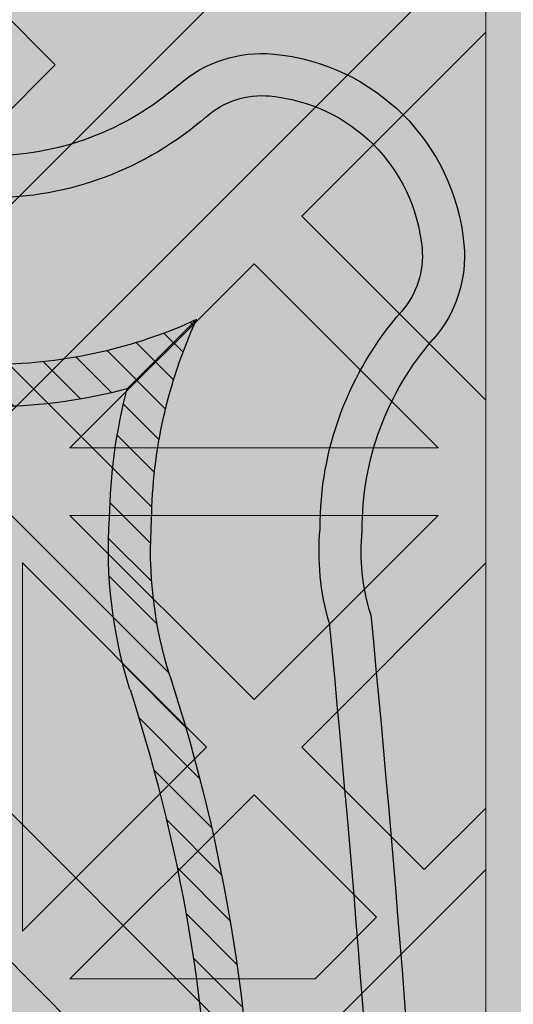
# Model space of a CAD drawing. Units: inches. Extents: x 844 to 2234, y 346 to 1084.
# Tile 86 of 93: x 2006.557 to 2008.425, y 706.497 to 710.224. Entities that reach past the tile are written whole.
import ezdxf

# ---------------------------------------------------------------- set-up
doc = ezdxf.new("R2010")
doc.units = ezdxf.units.IN
doc.header["$MEASUREMENT"] = 0
for name, color, linetype, lineweight in [('A-ANNO-DIMS', 2, 'Continuous', 18), ('furniture', 8, 'Continuous', 18), ('RA-AP-01$0$INT', 35, 'Continuous', 5)]:
    doc.layers.add(name, color=color, linetype=linetype, lineweight=lineweight)
doc.layers.add('RA-AP-01$0$FURN', color=3, linetype='Continuous')
doc.layers.add('RA-AP-01$0$WOOD', color=64, linetype='Continuous')
doc.styles.get("Standard").update_dxf_attribs({"font": 'arial.ttf'})
doc.dimstyles.get("Standard").update_dxf_attribs({"dimtxt": 6, "dimasz": 3, "dimexe": 0.18, "dimexo": 0.0625, "dimgap": 0.09, "dimtad": 0, "dimtih": 1, "dimtoh": 1, "dimdec": 1, "dimzin": 0, "dimdsep": 46, "dimlunit": 3, "dimtxsty": 'Standard', "dimblk": 'ARCHTICK', "dimcen": 0.09, "dimadec": 0, "dimazin": 0, "dimtfac": 1, "dimtdec": 1, "dimtofl": 0, "dimtmove": 0, "dimatfit": 3, "dimfxl": 1, "dimtolj": 1, "dimtzin": 0, "dimarcsym": 0})

# ---------------------------------------------------------------- blocks, each defined once
blk = doc.blocks.new('A$C18D01794')
at = {"layer": 'RA-AP-01$0$INT'}
blk.add_hatch(color=256, dxfattribs=at).paths.add_polyline_path([(4.505206456958071, -7.906712009588039), (5.305206456958072, -7.906712009588039), (5.305206456958072, -7.106712009588038), (5.255206456951893, -7.106712009588036), (5.25520645694868, -7.856712009570104), (4.555206456959269, -7.856712009588616), (4.555206456956052, -7.106712009588038), (4.505206456958073, -7.106712009588038)])
h = blk.add_hatch(color=256, dxfattribs=at)
h.paths.add_polyline_path([(4.585917135068448, -7.856712009587804), (4.614201406330596, -7.856712009587056), (4.668846067270487, -7.802067348644738), (4.723490728212344, -7.856712009584164), (4.771774999457151, -7.856712009582887), (4.826419660396886, -7.80206734864072), (4.862780050090322, -7.838427738332541), (4.844495778842715, -7.856712009580965), (4.862780050090411, -7.856712009580482), (4.905206456960182, -7.814285602707865), (4.947632863832445, -7.856712009578238), (4.965917135079675, -7.856712009577755), (4.947632863831759, -7.838427738330656), (4.983993253523576, -7.802067348637219), (5.038637914464627, -7.856712009575829), (5.08692218571208, -7.856712009574554), (5.141566846649976, -7.802067348634224), (5.196211507589851, -7.856712009571666), (5.224495778822615, -7.856712009570916), (4.905206456953975, -7.537422687702283)])
h.paths.add_polyline_path([(4.895206456956031, -7.575706958950402), (4.895206456958921, -7.684996280828174), (4.840561796018589, -7.630351619890275)], flags=16)
h.paths.add_polyline_path([(4.915206456955638, -7.575706958949956), (4.969851117895509, -7.630351619887399), (4.915206456957609, -7.684996280827732)], flags=16)
h.paths.add_polyline_path([(4.826419660395175, -7.644493755514321), (4.881064321335613, -7.699138416452331), (4.771774999456703, -7.69913841645522)], flags=16)
h.paths.add_polyline_path([(4.983993253519558, -7.644493755510815), (5.038637914460456, -7.699138416449285), (4.929348592581548, -7.69913841645126)], flags=16)
h.paths.add_polyline_path([(4.881064321336025, -7.719138416452334), (4.826419660397532, -7.773783077393256), (4.771774999457062, -7.719138416455217)], flags=16)
h.paths.add_polyline_path([(4.929348592582019, -7.71913841645126), (5.038637914460982, -7.719138416449284), (4.983993253522945, -7.773783077389749)], flags=16)
h.paths.add_polyline_path([(4.895206456960191, -7.733280552075633), (4.895206456962115, -7.806001331460164), (4.876922185715016, -7.824285602708492), (4.840561796021581, -7.787925213016675)], flags=16)
h.paths.add_polyline_path([(4.915206456958487, -7.733280552075187), (4.969851117899527, -7.787925213013798), (4.933490728206909, -7.824285602708034), (4.9152064569598, -7.806001331461736)], flags=16)
h.paths.add_polyline_path([(4.757632863832376, -7.733280552079264), (4.812277524772842, -7.787925213017304), (4.757632863834348, -7.842569873958233)], flags=16)
h.paths.add_polyline_path([(4.737632863832376, -7.73328055207979), (4.737632863834348, -7.842569873958701), (4.682988202893906, -7.787925213020692)], flags=16)
h.paths.add_polyline_path([(5.05278005008503, -7.733280552072701), (5.052780050087917, -7.842569873951664), (4.998135389146995, -7.787925213013169)], flags=16)
h.paths.add_polyline_path([(5.072780050085024, -7.733280552072333), (5.127424711025931, -7.787925213010806), (5.072780050087916, -7.842569873951244)], flags=16)
h.paths.add_polyline_path([(4.935917135072783, -7.506712009583784), (5.255206456948811, -7.826001331459767), (5.255206456948932, -7.797717060211899), (5.200561796010279, -7.743072399273238), (5.255206456949403, -7.688427738334128), (5.25520645694961, -7.640143467086677), (5.200561796009787, -7.585498806146837), (5.236922185702417, -7.549138416454212), (5.255206456949919, -7.56742268770172), (5.255206456949998, -7.549138416454178), (5.212780050078687, -7.506712009583814), (5.25520645695036, -7.464285602712145), (5.255206456950438, -7.446001331464763), (5.236922185702424, -7.464285602712779), (5.200561796009796, -7.427925213020149), (5.255206456950753, -7.373280552079203), (5.25520645695096, -7.324996280834394), (5.200561796010322, -7.270351619893748), (5.255206456951428, -7.215706958952649), (5.255206456951547, -7.187422687705071)])
h.paths.add_polyline_path([(5.042988202883395, -7.42792521302065), (5.097632863823085, -7.373280552080975), (5.097632863822622, -7.482569873959883)], flags=16)
h.paths.add_polyline_path([(5.028846067259663, -7.442067348644384), (5.083490728198774, -7.496712009583504), (4.974201406321001, -7.496712009583035)], flags=16)
h.paths.add_polyline_path([(5.117632863823087, -7.37328055208089), (5.172277524762331, -7.42792521302015), (5.11763286382262, -7.482569873959851)], flags=16)
h.paths.add_polyline_path([(5.08349072819877, -7.516712009582191), (5.028846067259652, -7.571356670521302), (4.974201406320998, -7.516712009582638)], flags=16)
h.paths.add_polyline_path([(5.131774999446817, -7.35913841645716), (5.186419660386065, -7.413783077396415), (5.241064321325782, -7.359138416456712)], flags=17)
h.paths.add_polyline_path([(5.131774999446228, -7.496712009583703), (5.186419660386065, -7.442067348643883), (5.222780050079488, -7.478427738337313), (5.204495778832781, -7.496712009584014)], flags=16)
h.paths.add_polyline_path([(5.097632863822613, -7.530854145205813), (5.097632863823061, -7.640143467084723), (5.042988202883383, -7.585498806145032)], flags=16)
h.paths.add_polyline_path([(5.131774999446899, -7.339138416457162), (5.241064321325809, -7.339138416456712), (5.186419660386591, -7.284493755517479)], flags=17)
h.paths.add_polyline_path([(5.131774999446226, -7.516712009581999), (5.204495778830767, -7.516712009581702), (5.22278005007868, -7.534996280829206), (5.186419660386049, -7.571356670521828)], flags=16)
h.paths.add_polyline_path([(5.11763286382262, -7.530854145205852), (5.17227752476232, -7.585498806145562), (5.117632863823064, -7.64014346708481)], flags=16)
h.paths.add_polyline_path([(5.186419660386069, -7.599640941770585), (5.241064321325754, -7.654285602710281), (5.131774999446791, -7.654285602709814)], flags=16)
h.paths.add_polyline_path([(5.131774999446872, -7.674285602709813), (5.24106432132578, -7.674285602710282), (5.186419660386554, -7.728930263649504)], flags=16)
h.paths.add_polyline_path([(5.255206456951811, -7.126001331467467), (5.255206456951895, -7.106712009588038), (4.555206456956052, -7.106712009588038), (4.555206456956136, -7.12600133146746), (4.905206456953973, -7.476001331465289)])
h.paths.add_polyline_path([(4.983993253513404, -7.368930263651977), (4.92934859257295, -7.314285602713969), (5.03863791445186, -7.314285602711063)], flags=16)
h.paths.add_polyline_path([(4.969851117889988, -7.383072399276016), (4.915206456952556, -7.437717060215906), (4.915206456949648, -7.328427738338133)], flags=16)
h.paths.add_polyline_path([(4.929348592572535, -7.294285602713971), (4.983993253511019, -7.239640941773039), (5.038637914451496, -7.294285602711065)], flags=16)
h.paths.add_polyline_path([(5.052780050074912, -7.280143467087016), (4.998135389134438, -7.225498806148989), (5.052780050072919, -7.170854145208052)], flags=16)
h.paths.add_polyline_path([(5.07278005007491, -7.280143467086489), (5.072780050072918, -7.170854145207579), (5.127424711013374, -7.225498806145578)], flags=16)
h.paths.add_polyline_path([(4.89520645695295, -7.437717060216355), (4.840561796013067, -7.383072399278919), (4.895206456950961, -7.328427738338582)], flags=16)
h.paths.add_polyline_path([(4.915206456948365, -7.280143467090674), (4.915206456946434, -7.207422687704125), (4.933490728192729, -7.18913841645701), (4.969851117886972, -7.225498806149623)], flags=16)
h.paths.add_polyline_path([(4.881064321327021, -7.314285602715054), (4.82641966038902, -7.368930263655506), (4.771774999448108, -7.314285602717047)], flags=16)
h.paths.add_polyline_path([(4.895206456950073, -7.280143467091125), (4.840561796009022, -7.225498806152518), (4.876922185700835, -7.18913841645908), (4.895206456948749, -7.207422687706589)], flags=16)
h.paths.add_polyline_path([(4.983993253510392, -7.211356670525576), (4.947632863816944, -7.174996280833758), (4.965917135064043, -7.156712009585847), (5.038637914448995, -7.156712009584522)], flags=16)
h.paths.add_polyline_path([(4.881064321326543, -7.294285602715056), (4.771774999447578, -7.294285602717046), (4.826419660385607, -7.239640941776569)], flags=16)
h.paths.add_polyline_path([(4.905206456946447, -7.19913841645844), (4.862780050074785, -7.156712009587725), (4.947632863816685, -7.156712009586302)], flags=16)
h.paths.add_polyline_path([(5.14156684663679, -7.211356670521528), (5.086922185696452, -7.156712009583639), (5.196211507574223, -7.156712009581651)], flags=16)
h.paths.add_polyline_path([(4.8264196603837, -7.211356670529104), (4.771774999442643, -7.156712009590501), (4.8444957788276, -7.156712009588568), (4.862780050075511, -7.17499628083566)], flags=16)
h.paths.add_polyline_path([(4.812277524760289, -7.225498806153156), (4.757632863822258, -7.28014346709363), (4.757632863819352, -7.170854145214669)], flags=16)
h.paths.add_polyline_path([(4.73763286382226, -7.280143467093997), (4.682988202881349, -7.22549880615554), (4.737632863819352, -7.170854145215086)], flags=16)
h.paths.add_polyline_path([(4.723490728195188, -7.156712009591787), (4.668846067257299, -7.211356670532127), (4.614201406317417, -7.156712009594693)], flags=16)
h.paths.add_polyline_path([(4.597632863829262, -7.506712009583814), (4.555206456957951, -7.54913841645418), (4.555206456958029, -7.56742268770172), (4.573490728205535, -7.549138416454212), (4.609851117898167, -7.585498806146839), (4.555206456958338, -7.640143467086675), (4.555206456958546, -7.688427738334125), (4.60985111789767, -7.743072399273238), (4.555206456959015, -7.797717060211899), (4.555206456959138, -7.826001331459767), (4.874495778835167, -7.506712009583786), (4.5552064569564, -7.187422687705062), (4.555206456956523, -7.215706958952644), (4.609851117897629, -7.270351619893746), (4.555206456956988, -7.324996280834396), (4.555206456957198, -7.373280552079195), (4.609851117898153, -7.427925213020147), (4.573490728205528, -7.464285602712779), (4.555206456957507, -7.446001331464756), (4.555206456957585, -7.464285602712143)])
h.paths.add_polyline_path([(4.712780050085332, -7.482569873959882), (4.712780050084863, -7.373280552080972), (4.767424711024555, -7.42792521302065)], flags=16)
h.paths.add_polyline_path([(4.726922185709173, -7.496712009583504), (4.781566846648288, -7.442067348644384), (4.836211507586949, -7.496712009583033)], flags=16)
h.paths.add_polyline_path([(4.692780050085327, -7.482569873959851), (4.638135389145619, -7.427925213020149), (4.692780050084865, -7.373280552080892)], flags=16)
h.paths.add_polyline_path([(4.726922185709182, -7.516712009582191), (4.836211507586949, -7.51671200958264), (4.7815668466483, -7.571356670521304)], flags=16)
h.paths.add_polyline_path([(4.678637914461726, -7.496712009583706), (4.605917135075169, -7.496712009584014), (4.587632863828464, -7.478427738337311), (4.623993253521887, -7.442067348643881)], flags=16)
h.paths.add_polyline_path([(4.712780050085336, -7.530854145205816), (4.767424711024568, -7.585498806145034), (4.71278005008489, -7.640143467084724)], flags=16)
h.paths.add_polyline_path([(4.678637914461726, -7.516712009582001), (4.623993253521899, -7.571356670521829), (4.587632863829271, -7.534996280829206), (4.605917135077185, -7.5167120095817)], flags=16)
h.paths.add_polyline_path([(4.692780050085336, -7.530854145205848), (4.692780050084889, -7.64014346708481), (4.638135389145632, -7.585498806145562)], flags=16)
h.paths.add_polyline_path([(4.623993253521885, -7.413783077396415), (4.678637914461131, -7.359138416457161), (4.56934859258217, -7.359138416456712)], flags=17)
h.paths.add_polyline_path([(4.623993253521901, -7.599640941770568), (4.678637914461158, -7.654285602709814), (4.569348592582195, -7.654285602710281)], flags=16)
h.paths.add_polyline_path([(4.678637914461051, -7.339138416457162), (4.623993253521361, -7.284493755517479), (4.569348592582143, -7.339138416456712)], flags=17)
h.paths.add_polyline_path([(4.678637914461076, -7.674285602709813), (4.623993253521399, -7.728930263649504), (4.569348592582167, -7.674285602710281)], flags=16)
h = blk.add_hatch(color=256, dxfattribs=at)
h.paths.add_polyline_path([(4.905206456954232, -7.537422687702028), (4.874495778835232, -7.506712009583718), (4.555206456959138, -7.826001331459766), (4.555206456959269, -7.856712009588616), (4.585917135068449, -7.856712009587804)])
h.paths.add_polyline_path([(4.935917135072152, -7.506712009583152), (4.905206456953497, -7.537422687701806), (5.224495778822614, -7.856712009570917), (5.255206456948681, -7.856712009570104), (5.255206456948813, -7.826001331459768)])
h.paths.add_polyline_path([(5.255206456951549, -7.18742268770507), (5.255206456951813, -7.126001331467461), (4.905206456953563, -7.476001331465701), (4.935917135072559, -7.506712009584006)])
h.paths.add_polyline_path([(4.874495778835167, -7.506712009583785), (4.905206456953818, -7.476001331465132), (4.555206456956135, -7.126001331467458), (4.555206456956399, -7.187422687705064)])
h = blk.add_hatch(color=256, dxfattribs=at)
h.paths.add_polyline_path([(4.781566846647504, -7.442067348645805), (4.836211507586161, -7.496712009584463), (4.726922185708388, -7.496712009584918)])
h.paths.add_polyline_path([(4.836211507586161, -7.516712009584068), (4.781566846647504, -7.571356670522723), (4.726922185708388, -7.516712009583606)])
h.paths.add_polyline_path([(4.76742471102377, -7.585498806146453), (4.712780050084083, -7.640143467086137), (4.712780050084542, -7.530854145207227)])
h.paths.add_polyline_path([(4.692780050084544, -7.530854145207257), (4.692780050084084, -7.64014346708622), (4.638135389144834, -7.585498806146965)])
h.paths.add_polyline_path([(4.678637914460932, -7.516712009583407), (4.623993253521102, -7.571356670523233), (4.587632863827676, -7.53499628082981), (4.605917135074382, -7.516712009583104)])
h.paths.add_polyline_path([(4.573490728204743, -7.54913841645434), (4.60985111789737, -7.585498806146969), (4.555206456957541, -7.640143467086797), (4.555206456957237, -7.567422687701846)])
h.paths.add_polyline_path([(4.623993253521098, -7.599640941770699), (4.67863791446035, -7.654285602709951), (4.56934859258139, -7.654285602710407)])
h.paths.add_polyline_path([(4.678637914460275, -7.67428560270995), (4.623993253520583, -7.728930263649637), (4.56934859258136, -7.674285602710405)])
h.paths.add_polyline_path([(4.609851117896854, -7.743072399273369), (4.555206456958196, -7.797717060212026), (4.555206456957738, -7.688427738334254)])
h.paths.add_polyline_path([(4.597632863828475, -7.506712009583301), (4.555206456957283, -7.549138416454495), (4.555206456956805, -7.464285602712587)])
h.paths.add_polyline_path([(4.678637914460932, -7.496712009585113), (4.605917135076396, -7.496712009585417), (4.587632863828479, -7.478427738337913), (4.623993253521104, -7.442067348645284)])
h.paths.add_polyline_path([(4.692780050084091, -7.373280552082301), (4.692780050084548, -7.482569873961267), (4.638135389144834, -7.427925213021552)])
h.paths.add_polyline_path([(4.767424711023772, -7.427925213022072), (4.712780050084545, -7.48256987396129), (4.712780050084089, -7.373280552082384)])
h.paths.add_polyline_path([(4.67863791446036, -7.359138416457298), (4.623993253521105, -7.41378307739655), (4.569348592581399, -7.35913841645684)])
h.paths.add_polyline_path([(4.609851117897371, -7.427925213020278), (4.573490728204743, -7.464285602712907), (4.555206456957237, -7.446001331465401), (4.555206456957548, -7.373280552080448)])
h.paths.add_polyline_path([(4.623993253520596, -7.284493755517612), (4.67863791446028, -7.339138416457299), (4.569348592581367, -7.339138416456838)])
h.paths.add_polyline_path([(4.609851117896867, -7.270351619893878), (4.555206456957749, -7.324996280832994), (4.55520645695821, -7.21570695895522)])
h = blk.add_hatch(color=256, dxfattribs=at)
h.paths.add_polyline_path([(4.969851117891331, -7.630351619889621), (4.915206456952669, -7.575706958950966), (4.915206456952222, -7.684996280828739)])
h.paths.add_polyline_path([(4.895206456953064, -7.575706958950968), (4.840561796014413, -7.630351619889628), (4.895206456953533, -7.684996280828741)])
h.paths.add_polyline_path([(4.826419660390684, -7.644493755513362), (4.771774999451003, -7.699138416453052), (4.881064321329913, -7.699138416452587)])
h.paths.add_polyline_path([(4.881064321329884, -7.719138416452585), (4.771774999450921, -7.719138416453052), (4.82641966039018, -7.773783077392298)])
h.paths.add_polyline_path([(4.895206456953734, -7.733280552076196), (4.840561796013912, -7.787925213016031), (4.876922185707337, -7.824285602709455), (4.895206456954043, -7.806001331462747)])
h.paths.add_polyline_path([(4.862780050082808, -7.838427738332388), (4.826419660390178, -7.802067348639763), (4.771774999450351, -7.856712009579595), (4.844495778835303, -7.856712009579895)])
h.paths.add_polyline_path([(4.812277524766446, -7.787925213016036), (4.757632863827191, -7.733280552076788), (4.757632863826741, -7.842569873955747)])
h.paths.add_polyline_path([(4.737632863827191, -7.733280552076863), (4.682988202887508, -7.787925213016558), (4.737632863826743, -7.842569873955778)])
h.paths.add_polyline_path([(4.668846067263777, -7.802067348640287), (4.614201406325123, -7.856712009578949), (4.723490728202894, -7.856712009579402)])
h.paths.add_polyline_path([(4.905206456953846, -7.814285602708654), (4.862780050082654, -7.856712009579847), (4.947632863824561, -7.85671200958032)])
h.paths.add_polyline_path([(4.915206456952028, -7.733280552076195), (4.91520645695173, -7.806001331460731), (4.933490728199234, -7.824285602708648), (4.96985111789186, -7.787925213016022)])
h.paths.add_polyline_path([(5.038637914454841, -7.719138416453029), (4.929348592575874, -7.71913841645258), (4.983993253515593, -7.773783077392289)])
h.paths.add_polyline_path([(4.983993253515065, -7.644493755513352), (4.929348592575849, -7.699138416452582), (5.038637914454755, -7.699138416453031)])
h.paths.add_polyline_path([(5.052780050079843, -7.73328055207676), (4.998135389140595, -7.787925213016018), (5.052780050080309, -7.842569873955721)])
h.paths.add_polyline_path([(4.983993253516868, -7.802067348639752), (4.947632863824241, -7.838427738332383), (4.965917135071747, -7.856712009579888), (5.038637914456701, -7.856712009579572)])
h.paths.add_polyline_path([(5.127424711019533, -7.787925213016519), (5.072780050079843, -7.733280552076838), (5.07278005008031, -7.842569873955751)])
h.paths.add_polyline_path([(5.141566846643269, -7.802067348640248), (5.086922185704154, -7.85671200957937), (5.196211507581929, -7.856712009578901)])
for p, q in [((4.555206456956052, -7.106712009588036), (4.555206456959269, -7.856712009588616)), ((4.55520645695807, -7.464285602712626), (4.555206456957598, -7.549138416454534)), ((4.597632863829264, -7.506712009583814), (4.555206456957598, -7.549138416454534)), ((4.874495778835167, -7.506712009583786), (4.555206456959136, -7.826001331459769)), ((4.605917135074869, -7.516712009584017), (4.587632863829269, -7.534996280829206)), ((4.605917135076771, -7.5167120095817), (4.678637914461723, -7.516712009581999)), ((4.678637914461723, -7.516712009581999), (4.623993253521898, -7.571356670521829)), ((4.692780050085336, -7.530854145205847), (4.638135389145632, -7.585498806145562)), ((4.692780050084889, -7.64014346708481), (4.692780050085336, -7.530854145205847)), ((4.623993253521899, -7.571356670521829), (4.587632863829269, -7.534996280829206)), ((4.905206456953975, -7.537422687702283), (4.585917135071132, -7.856712009585121)), ((4.555206456958031, -7.56742268770172), (4.573490728205535, -7.549138416454212)), ((4.609851117898167, -7.585498806146839), (4.573490728205535, -7.549138416454214)), ((4.555206456958033, -7.56742268770172), (4.555206456958345, -7.640143467086671)), ((4.555206456958345, -7.640143467086671), (4.609851117898167, -7.585498806146837)), ((4.692780050084889, -7.64014346708481), (4.638135389145632, -7.585498806145562)), ((4.569348592582195, -7.654285602710281), (4.623993253521901, -7.599640941770568)), ((4.678637914461158, -7.654285602709814), (4.623993253521901, -7.599640941770568)), ((4.678637914461158, -7.654285602709814), (4.569348592582195, -7.654285602710281)), ((4.569348592582168, -7.674285602710281), (4.623993253521399, -7.728930263649504)), ((4.678637914461078, -7.674285602709813), (4.569348592582168, -7.674285602710281)), ((4.6239932535214, -7.728930263649502), (4.678637914461078, -7.674285602709813)), ((4.555206456958551, -7.68842773833413), (4.60985111789767, -7.743072399273238)), ((4.682988202893908, -7.78792521302069), (4.737632863832376, -7.733280552079792)), ((4.555206456959017, -7.797717060211899), (4.60985111789767, -7.743072399273238)), ((4.737632863834348, -7.842569873958701), (4.682988202893906, -7.787925213020692))]:
    blk.add_line(p, q, dxfattribs=at)
blk = doc.blocks.new('A$C32926AE1')
at = {"layer": 'RA-AP-01$0$WOOD'}
h = blk.add_hatch(color=256, dxfattribs=at)
h.dxf.hatch_style = 1
h.paths.add_polyline_path([(5.157430609644524, 4.573483066760929, -0.1009492694046607), (5.155401577623758, 4.593365984175333, -0.1842662638101597), (5.172249623284174, 4.638795604568598, 0.2056608120311276), (5.179560981299304, 4.661316324430096, 0.3614336704623542), (5.134352340494423, 4.706524965234944, 0.2056608120311297), (5.111831620632933, 4.699213607219793, -0.1842662638101113), (5.066402000239693, 4.682365561559342, -0.1055311479399994), (5.045656153913092, 4.68467289944697, 0.1567636581983829), (4.763886414745334, 4.684672899446966, -0.1055311479399895), (4.743140568418733, 4.68236556155934, -0.1842662638100833), (4.6977109480255, 4.69921360721979, 0.2056608120302612), (4.675190228164109, 4.706524965234949, 0.3614336704708441), (4.629981587358889, 4.66131632442871, 0.2056608120245944), (4.637292945374126, 4.638795604567974, -0.1842662638101024), (4.654140991034615, 4.59336598417475, -0.1009492694055169), (4.652111959013835, 4.573483066760181, 0.021410119221476), (4.629748025606143, 4.156712009541676, 0.0214101192214795), (4.652111959013809, 3.739940952323101, -0.1009492694059586), (4.654140991034615, 3.720058034908448, -0.1842662638100975), (4.637292945374126, 3.674628414515226, 0.2056608120245705), (4.629981587358889, 3.652107694654492, 0.3614336704708879), (4.675190228164113, 3.606899053848249, 0.2056608120302384), (4.697710948025501, 3.614210411863408, -0.1842662638100995), (4.743140568418738, 3.63105845752386, -0.1055311479402541), (4.763886414745388, 3.628751119636215, 0.1567636581983776), (5.045656153913137, 3.628751119636244, -0.1055311479397538), (5.066402000239692, 3.631058457523857, -0.1842662638101067), (5.111831620632931, 3.614210411863407, 0.2056608120310924), (5.134352340494417, 3.606899053848256, 0.3614336704624001), (5.179560981299307, 3.652107694653103, 0.2056608120311314), (5.172249623284175, 3.6746284145146, -0.1842662638101402), (5.155401577623758, 3.72005803490786, -0.1009492694051366), (5.15743060964455, 3.739940952322354, 0.0214101192215073), (5.179794543052287, 4.156712009541468, 0.0214101192215252)])
h.paths.add_polyline_path([(4.639748609479751, 4.156712009541513, 0.0213537860821624), (4.661970494867118, 3.741887061152232, -0.094075836301374), (4.664143710413708, 3.7196126951003, -0.1824818158568985), (4.644813765429836, 3.668037719127816, 0.2056608120245319), (4.639939526753007, 3.653023905887301, 0.3614336704710246), (4.676106439397173, 3.616856993242342, 0.2056608120302234), (4.691120252638095, 3.621731231919122, -0.1824818158602558), (4.742695228611606, 3.641061176902986, -0.1029891339458722), (4.766991894714349, 3.638256818950944, 0.156709409989566), (5.042550673941472, 3.638256818950105, -0.102989133958497), (5.066847340047078, 3.641061176902949, -0.1824818158594995), (5.118422316020358, 3.621731231919103, 0.2056608120311416), (5.133436129261316, 3.616856993242346, 0.3614336704621468), (5.169603041905217, 3.653023905886178, 0.2056608120310986), (5.164728803228477, 3.668037719127177, -0.1824818158565612), (5.145398858244737, 3.719612695099578, -0.0940758363009313), (5.147572073791232, 3.741887061151398, 0.0213537860822023), (5.169793959178681, 4.156712009541451, 0.0213537860822226), (5.147572073791203, 4.571536957931898, -0.0940758363005034), (5.145398858244737, 4.59381132398362, -0.1824818158565587), (5.164728803228476, 4.645386299956021, 0.2056608120311045), (5.169603041905216, 4.66040011319702, 0.3614336704621845), (5.133436129261313, 4.696567025840856, 0.2056608120310773), (5.118422316020359, 4.691692787164098, -0.182481815859508), (5.066847340047078, 4.67236284218025, -0.1029891339584606), (5.04255067394148, 4.675167200133092, 0.156709409989566), (4.766991894714357, 4.675167200132257, -0.1029891339458842), (4.742695228611611, 4.672362842180213, -0.1824818158602725), (4.691120252638095, 4.691692787164077, 0.2056608120302152), (4.676106439397174, 4.696567025840858, 0.3614336704710363), (4.639939526753005, 4.660400113195899, 0.2056608120245495), (4.644813765429837, 4.645386299955384, -0.1824818158568934), (4.664143710413708, 4.593811323982902, -0.0940758363009187), (4.661970494867149, 4.571536957931074, 0.021353786082177)], flags=16)
h.paths.add_polyline_path([(5.129794543052235, 4.432167055276933, -0.0141661062790638), (5.130152669293814, 4.156927903047693, -0.0141661062790647), (5.129794543052234, 3.881688750818433, -0.0785247771143638), (5.10979738006795, 3.755143611847103, 0.0945969212073497), (5.105408519571111, 3.717898134952927, 0.1043170707844957), (5.116074640131521, 3.670385395016088, 0.1043170707864965), (5.068561900193738, 3.681051515576561, 0.09459692119553), (5.031316423304057, 3.676662655080835, -0.1580239521427272), (4.778226145355827, 3.676662655080367, 0.0945969211986668), (4.740980668464973, 3.681051515576592, 0.1043170707882822), (4.693467928526415, 3.670385395015844, 0.1043170707867916), (4.704134049087309, 3.717898134953662, 0.0945969211972894), (4.69974518859162, 3.755143611844042, -0.0785247771163196), (4.679748025606343, 3.881688750818406, -0.0141661062790663), (4.679389899364763, 4.156927903047693, -0.0141661062790672), (4.679748025606343, 4.432167055276998, -0.0785247771163064), (4.699745188591625, 4.55871219425134, 0.094596921197333), (4.704134049087308, 4.595957671141738, 0.1043170707867205), (4.693467928526416, 4.643470411079523, 0.1043170707882628), (4.740980668464965, 4.632804290518776, 0.0945969211988114), (4.778226145355874, 4.637193151015016, -0.158023952142669), (5.031316423304015, 4.637193151014546, 0.0945969211956361), (5.068561900193736, 4.632804290518806, 0.1043170707864979), (5.11607464013152, 4.643470411079278, 0.1043170707844617), (5.105408519571112, 4.595957671142455, 0.0945969212074597), (5.109797380067959, 4.558712194248236, -0.0785247771143467)], flags=0)
h.paths.add_polyline_path([(5.119794532311105, 4.432259799204851, -0.0142000800617244), (5.120156169157484, 4.156927903047701, -0.0142000800617277), (5.119794532311105, 3.881596006890482, -0.0784894509520253), (5.100273383573699, 3.758192358677797, 0.0940138827242913), (5.095413455884425, 3.717477693979438, 0.0606271852308753), (5.099615656341024, 3.686844378806616, 0.0606271852322524), (5.068982341167493, 3.691046579263239, 0.0940138827010453), (5.028267676478798, 3.686186651576848, -0.1580706864508061), (4.781274892180912, 3.686186651576435, 0.0940138827026903), (4.740560227491556, 3.691046579263279, 0.0606271852339895), (4.709926912317155, 3.686844378806508, 0.0606271852329405), (4.714129112773991, 3.717477693980356, 0.094013882701304), (4.709269185087677, 3.758192358669163, -0.0784894509577193), (4.689748036347473, 3.881596006890469, -0.014200080061729), (4.689386399501094, 4.156927903047709, -0.0142000800617217), (4.689748036347473, 4.432259799204808, -0.078489450957724), (4.709269185087651, 4.555663447426125, 0.0940138827014585), (4.714129112773992, 4.596378112114996, 0.0606271852329731), (4.709926912317154, 4.62701142728886, 0.0606271852340196), (4.74056022749157, 4.622809226832087, 0.0940138827024997), (4.781274892180847, 4.627669154518912, -0.1580706864508359), (5.028267676478777, 4.627669154518526, 0.0940138827010946), (5.068982341167492, 4.622809226832129, 0.060627185232254), (5.099615656341024, 4.627011427288751, 0.0606271852308727), (5.095413455884425, 4.59637811211593, 0.0940138827241088), (5.100273383573675, 4.555663447417647, -0.0784894509520978)], flags=0)
h.paths.add_polyline_path([(5.06978912287499, 4.430218106756144, -0.014241683694547), (5.070173729147532, 4.156927903047672, -0.0142416836945458), (5.06978912287499, 3.883637699339223, -0.0800609523125196), (5.052662118612511, 3.773463122773442, 0.0526421978001116), (5.04590916754064, 3.740550867606997, 0.0526421977992423), (5.012996912374707, 3.73379791653534, -0.1583028414718258), (4.796545656286308, 3.73379791653451, 0.0526421978034211), (4.763633401117837, 3.740550867607021, 0.0526421978018622), (4.756880450045755, 3.773463122774558, -0.0800609523117106), (4.739753445783639, 3.883637699339268, -0.0142416836945435), (4.739368839511098, 4.156927903047671, -0.0142416836945477), (4.739753445783639, 4.430218106756155, -0.0800609523116345), (4.75688045004574, 4.540392683320762, 0.052642197801941), (4.763633401117837, 4.573304938488346, 0.0526421978035071), (4.796545656286361, 4.580057889560873, -0.1583028414717561), (5.012996912374669, 4.580057889560039, 0.0526421977993048), (5.04590916754064, 4.57330493848837, 0.0526421978002057), (5.052662118612529, 4.540392683321868, -0.080060952312477)], flags=0)
h.paths.add_polyline_path([(5.049789715110557, 4.43038092723357, -0.0143097550741839), (5.05018085590259, 4.156927903047715, -0.0143097550741854), (5.049789715110558, 3.883474878861827, -0.0800685599149176), (5.03362098255317, 3.779581877367999, 0.0306258898956367), (5.028241146483733, 3.758218888663947, 0.0306258898977031), (5.006878157778253, 3.75283905259408, -0.1583983521624096), (4.802664410878162, 3.752839052594731, 0.0306258898946014), (4.781301422174808, 3.758218888663924, 0.0306258898967912), (4.775921586105202, 3.779581877368794, -0.080068559914251), (4.759752853548071, 3.883474878861786, -0.0143097550741854), (4.759361712756037, 4.156927903047671, -0.0143097550741854), (4.759752853548071, 4.430380927233557, -0.0800685599142479), (4.775921586105193, 4.534273928726546, 0.0306258898968306), (4.781301422174808, 4.555636917431444, 0.0306258898945754), (4.802664410878143, 4.561016753500631, -0.1583983521624168), (5.006878157778244, 4.561016753501291, 0.0306258898977177), (5.028241146483733, 4.555636917431421, 0.0306258898958182), (5.03362098255321, 4.534273928727244, -0.080068559914796)], flags=0)
h.paths.add_polyline_path([(4.999766070382627, 4.428171244713864, -0.0143443147609634), (5.000198441819402, 4.156927903047689, -0.0143443147609612), (4.999766070382627, 3.885684561381556, -0.0784641635803329), (4.987356730658798, 3.799103304488872, -0.1506053783831347), (4.822185837999821, 3.79910330448882, -0.0784641635803318), (4.809776498276007, 3.885684561381509, -0.014344314760963), (4.809344126839227, 4.156927903047677, -0.0143443147609645), (4.809776498276007, 4.428171244713873, -0.0784641635803192), (4.822185837999822, 4.514752501606549, -0.1506053783831338), (4.987356730658798, 4.514752501606494, -0.078464163580285)], flags=0)
h.paths.add_polyline_path([(4.979755254238824, 4.42764379880488, -0.0143772539198268), (4.980205517789977, 4.156927903047693, -0.0143772539198275), (4.979755254238824, 3.886212007290489, -0.0689242507424422), (4.971183264704897, 3.815276770442801, -0.1296645318904179), (4.838359303953726, 3.815276770442746, -0.0689242507424186), (4.829787314419809, 3.886212007290419, -0.0143772539198292), (4.829337050868653, 4.156927903047653, -0.0143772539198325), (4.829787314419809, 4.427643798804946, -0.0689242507424211), (4.838359303953725, 4.498579035652621, -0.1296645318904187), (4.971183264704897, 4.498579035652565, -0.0689242507424401)], flags=0)
h = blk.add_hatch(color=256, dxfattribs=at)
h.dxf.hatch_style = 1
h.paths.add_polyline_path([(5.145398858244737, 4.59381132398362, -0.1824818158565616), (5.164728803228476, 4.645386299956021, 0.2056608120311045), (5.169603041905216, 4.66040011319702, 0.3614336704621845), (5.133436129261313, 4.696567025840856, 0.2056608120310773), (5.118422316020359, 4.691692787164098, -0.182481815859508), (5.066847340047078, 4.67236284218025, -0.1029891339584606), (5.04255067394148, 4.675167200133092, 0.156709409989566), (4.766991894714357, 4.675167200132257, -0.1029891339458842), (4.742695228611611, 4.672362842180213, -0.1824818158602725), (4.691120252638095, 4.691692787164077, 0.2056608120302152), (4.676106439397174, 4.696567025840858, 0.3614336704710363), (4.639939526753005, 4.660400113195899, 0.2056608120245495), (4.644813765429837, 4.645386299955384, -0.1824818158568934), (4.664143710413708, 4.593811323982902, -0.0940758363009187), (4.661970494867149, 4.571536957931074, 0.0213537860821772), (4.639748609479751, 4.156712009541507, 0.0213537860821625), (4.661970494867119, 3.741887061152226, -0.0940758363013071), (4.664143710413708, 3.719612695100309, -0.1824818158569294), (4.644813765429836, 3.668037719127816, 0.2056608120245319), (4.639939526753007, 3.653023905887301, 0.3614336704710246), (4.676106439397173, 3.616856993242342, 0.2056608120302234), (4.691120252638095, 3.621731231919122, -0.1824818158602558), (4.742695228611606, 3.641061176902986, -0.1029891339458722), (4.766991894714349, 3.638256818950944, 0.156709409989566), (5.042550673941472, 3.638256818950105, -0.102989133958497), (5.066847340047078, 3.641061176902949, -0.1824818158594995), (5.118422316020358, 3.621731231919103, 0.2056608120311416), (5.133436129261316, 3.616856993242346, 0.3614336704621468), (5.169603041905217, 3.653023905886178, 0.2056608120310986), (5.164728803228477, 3.668037719127177, -0.1824818158565612), (5.145398858244737, 3.719612695099578, -0.0940758363009313), (5.147572073791232, 3.741887061151398, 0.0213537860822023), (5.169793959178681, 4.156712009541451, 0.0213537860822226), (5.147572073791203, 4.571536957931898, -0.0940758363004996)])
h.paths.add_polyline_path([(5.109797380067958, 4.55871219424824, -0.0785247771143472), (5.129794543052234, 4.432167055276936, -0.0141661062790644), (5.130152669293814, 4.156927903047685, -0.014166106279066), (5.129794543052234, 3.881688750818401, -0.0785247771143517), (5.109797380067946, 3.755143611847092, 0.0945969212073132), (5.105408519571111, 3.717898134952929, 0.1043170707844995), (5.116074640131521, 3.670385395016088, 0.1043170707864965), (5.068561900193738, 3.681051515576561, 0.09459692119553), (5.031316423304057, 3.676662655080835, -0.1580239521427272), (4.778226145355827, 3.676662655080367, 0.0945969211986668), (4.740980668464973, 3.681051515576592, 0.1043170707882822), (4.693467928526415, 3.670385395015844, 0.1043170707867916), (4.704134049087309, 3.717898134953662, 0.0945969211972894), (4.69974518859162, 3.755143611844042, -0.0785247771163196), (4.679748025606343, 3.881688750818406, -0.0141661062790663), (4.679389899364763, 4.156927903047693, -0.0141661062790672), (4.679748025606343, 4.432167055276998, -0.0785247771163064), (4.699745188591625, 4.55871219425134, 0.094596921197333), (4.704134049087308, 4.595957671141738, 0.1043170707867205), (4.693467928526416, 4.643470411079523, 0.1043170707882628), (4.740980668464965, 4.632804290518776, 0.0945969211988114), (4.778226145355874, 4.637193151015016, -0.158023952142669), (5.031316423304015, 4.637193151014546, 0.0945969211956361), (5.068561900193736, 4.632804290518806, 0.1043170707864979), (5.11607464013152, 4.643470411079278, 0.1043170707844617), (5.105408519571112, 4.595957671142455, 0.0945969212074504)], flags=16)
h.paths.add_polyline_path([(5.100273383573655, 4.55566344741771, -0.0784894509521388), (5.119794532311105, 4.432259799204852, -0.0142000800617252), (5.120156169157484, 4.156927903047686, -0.014200080061726), (5.119794532311105, 3.881596006890502, -0.0784894509520446), (5.100273383573696, 3.758192358677786, 0.0940138827242721), (5.095413455884425, 3.717477693979436, 0.0606271852308692), (5.099615656341024, 3.686844378806616, 0.0606271852322522), (5.068982341167493, 3.691046579263239, 0.0940138827010453), (5.028267676478798, 3.686186651576848, -0.1580706864508061), (4.781274892180912, 3.686186651576435, 0.0940138827026903), (4.740560227491556, 3.691046579263279, 0.0606271852339895), (4.709926912317155, 3.686844378806508, 0.0606271852329405), (4.714129112773991, 3.717477693980356, 0.094013882701304), (4.709269185087677, 3.758192358669163, -0.0784894509577193), (4.689748036347473, 3.881596006890469, -0.014200080061729), (4.689386399501094, 4.156927903047709, -0.0142000800617217), (4.689748036347473, 4.432259799204808, -0.078489450957724), (4.709269185087651, 4.555663447426125, 0.0940138827014585), (4.714129112773992, 4.596378112114996, 0.0606271852329731), (4.709926912317154, 4.62701142728886, 0.0606271852340196), (4.74056022749157, 4.622809226832087, 0.0940138827024997), (4.781274892180847, 4.627669154518912, -0.1580706864508359), (5.028267676478777, 4.627669154518526, 0.0940138827010946), (5.068982341167492, 4.622809226832129, 0.060627185232254), (5.099615656341024, 4.627011427288751, 0.0606271852308727), (5.095413455884425, 4.59637811211593, 0.094013882723957)], flags=0)
h.paths.add_polyline_path([(5.04590916754064, 4.57330493848837, 0.0526421978002057), (5.052662118612529, 4.540392683321868, -0.0800609523124783), (5.06978912287499, 4.430218106756142, -0.0142416836945469), (5.070173729147532, 4.156927903047672, -0.0142416836945458), (5.06978912287499, 3.883637699339223, -0.0800609523125196), (5.052662118612511, 3.773463122773442, 0.0526421978001116), (5.04590916754064, 3.740550867606997, 0.0526421977992423), (5.012996912374707, 3.73379791653534, -0.1583028414718258), (4.796545656286308, 3.73379791653451, 0.0526421978034211), (4.763633401117837, 3.740550867607021, 0.0526421978018622), (4.756880450045755, 3.773463122774558, -0.0800609523117106), (4.739753445783639, 3.883637699339268, -0.0142416836945435), (4.739368839511098, 4.156927903047671, -0.0142416836945477), (4.739753445783639, 4.430218106756155, -0.0800609523116345), (4.75688045004574, 4.540392683320762, 0.052642197801941), (4.763633401117837, 4.573304938488346, 0.0526421978035071), (4.796545656286361, 4.580057889560873, -0.1583028414717561), (5.012996912374669, 4.580057889560039, 0.0526421977993048)], flags=0)
h.paths.add_polyline_path([(5.028241146483733, 4.555636917431422, 0.0306258898956949), (5.033620982553182, 4.534273928727329, -0.0800685599148649), (5.049789715110557, 4.430380927233569, -0.0143097550741839), (5.05018085590259, 4.156927903047715, -0.0143097550741854), (5.049789715110558, 3.883474878861827, -0.0800685599149176), (5.03362098255317, 3.779581877367999, 0.0306258898956367), (5.028241146483733, 3.758218888663947, 0.0306258898977031), (5.006878157778253, 3.75283905259408, -0.1583983521624096), (4.802664410878162, 3.752839052594731, 0.0306258898946014), (4.781301422174808, 3.758218888663924, 0.0306258898967912), (4.775921586105202, 3.779581877368794, -0.080068559914251), (4.759752853548071, 3.883474878861786, -0.0143097550741854), (4.759361712756037, 4.156927903047671, -0.0143097550741854), (4.759752853548071, 4.430380927233557, -0.0800685599142479), (4.775921586105193, 4.534273928726546, 0.0306258898968306), (4.781301422174808, 4.555636917431444, 0.0306258898945754), (4.802664410878143, 4.561016753500631, -0.1583983521624168), (5.006878157778244, 4.561016753501291, 0.0306258898977174)], flags=0)
h.paths.add_polyline_path([(4.987356730658798, 4.514752501606494, -0.0784641635803018), (4.999766070382627, 4.428171244713845, -0.0143443147609637), (5.000198441819402, 4.156927903047665, -0.0143443147609622), (4.999766070382628, 3.885684561381514, -0.0784641635802952), (4.987356730658797, 3.799103304488872, -0.1506053783831338), (4.822185837999821, 3.799103304488819, -0.0784641635803342), (4.809776498276007, 3.885684561381512, -0.0143443147609628), (4.809344126839227, 4.156927903047676, -0.0143443147609646), (4.809776498276007, 4.428171244713873, -0.0784641635803192), (4.822185837999822, 4.514752501606549, -0.1506053783831338)], flags=0)
h.paths.add_polyline_path([(4.971183264704897, 4.498579035652566, -0.0689242507424384), (4.979755254238824, 4.427643798804883, -0.0143772539198276), (4.980205517789977, 4.15692790304768, -0.0143772539198258), (4.979755254238823, 3.88621200729051, -0.0689242507424628), (4.971183264704897, 3.815276770442801, -0.129664531890417), (4.838359303953726, 3.815276770442746, -0.0689242507424186), (4.829787314419809, 3.886212007290419, -0.0143772539198292), (4.829337050868653, 4.156927903047653, -0.0143772539198325), (4.829787314419809, 4.427643798804946, -0.0689242507424211), (4.838359303953725, 4.498579035652621, -0.1296645318904187)], flags=0)
h = blk.add_hatch(dxfattribs=at)
h.set_pattern_fill('ANSI31', color=256, scale=0.05, style=0)
h.set_pattern_definition([(45, (0, 0), (-0.0044194173824159, 0.0044194173824159), [])])
h.paths.add_polyline_path([(5.130152669293814, 4.156927903047704, 0.0141661062790657), (5.129794543052234, 4.432167055276982, 0.0777827904001433), (5.110168979996553, 4.557559993161921, -0.0976515123401879), (5.105408519571111, 4.595957671142454, -0.1043170707844687), (5.116074640131522, 4.64347041107928), (5.099615656341024, 4.627011427288751, 0.0606271852308727), (5.095413455884425, 4.59637811211593, 0.0940138827241088), (5.100273383573675, 4.555663447417647, -0.0784894509520972), (5.119794532311105, 4.432259799204852, -0.0142000800617252), (5.120156169157484, 4.156927903047686, -0.014200080061726), (5.119794532311105, 3.881596006890502, -0.0784894509520446), (5.100273383573696, 3.758192358677786, 0.0940138827242721), (5.095413455884425, 3.717477693979436, 0.0606271852308692), (5.099615656341024, 3.686844378806616), (5.116074640131519, 3.67038539501609, -0.1043170707844594), (5.105408519571112, 3.717898134952912, -0.0976515123401594), (5.11016897999655, 3.756295812933435, 0.0777827904001654), (5.129794543052234, 3.881688750818409, 0.0141661062790665)])
h.paths.add_polyline_path([(5.030164222210597, 3.676291055149937, -0.0976515123472002), (5.068561900193739, 3.681051515576561, -0.1043170707864927), (5.116074640131521, 3.670385395016088), (5.099615656341024, 3.686844378806616, 0.0606271852322522), (5.068982341167493, 3.691046579263239, 0.0940138827010453), (5.028267676478798, 3.686186651576848, -0.1580706864508061), (4.781274892180912, 3.686186651576435, 0.0940138827026903), (4.740560227491556, 3.691046579263279, 0.0606271852339913), (4.709926912317154, 3.686844378806508), (4.693467928526416, 3.670385395015845, -0.1043170707882796), (4.740980668464973, 3.681051515576592, -0.0976515123427246), (4.779378346446416, 3.676291055150394, 0.156512506893803)])
h.paths.add_polyline_path([(4.689748036347473, 3.881596006890472, -0.014200080061729), (4.689386399501094, 4.156927903047712, -0.0142000800617195), (4.689748036347473, 4.432259799204768, -0.078489450957742), (4.709269185087648, 4.555663447426114, 0.0940138827014821), (4.714129112773992, 4.596378112114995, 0.0606271852329748), (4.709926912317154, 4.62701142728886), (4.693467928526414, 4.643470411079524, -0.1043170707867939), (4.704134049087309, 4.595957671141706, -0.09765151234893), (4.699373588660725, 4.557559993157876, 0.0777827903975372), (4.679748025606343, 4.432167055276987, 0.0141661062790675), (4.679389899364763, 4.156927903047675, 0.0141661062790641), (4.679748025606343, 3.88168875081843, 0.0777827903975637), (4.699373588660724, 3.756295812937497, -0.0976515123490278), (4.704134049087308, 3.717898134953629, -0.1043170707867196), (4.693467928526416, 3.670385395015845), (4.709926912317155, 3.686844378806508, 0.0606271852329413), (4.714129112773991, 3.717477693980357, 0.0940138827013084), (4.709269185087676, 3.758192358669166, -0.0784894509577192)])
h.paths.add_polyline_path([(4.779378346446434, 4.63756475094498, -0.0976515123427943), (4.740980668464964, 4.632804290518776, -0.1043170707882609), (4.693467928526416, 4.643470411079523), (4.709926912317154, 4.62701142728886, 0.0606271852340196), (4.74056022749157, 4.622809226832087, 0.0940138827024997), (4.781274892180847, 4.627669154518912, -0.1580706864508359), (5.028267676478777, 4.627669154518526, 0.0940138827010946), (5.068982341167492, 4.622809226832129, 0.060627185232254), (5.099615656341024, 4.627011427288751), (5.116074640131521, 4.643470411079279, -0.1043170707865022), (5.068561900193735, 4.632804290518806, -0.0976515123475899), (5.030164222210446, 4.637564750945479, 0.1565125068936924)])
h = blk.add_hatch(dxfattribs=at)
h.set_pattern_fill('ANSI32', color=256, scale=0.2, style=0)
h.set_pattern_definition([(45, (0, 0), (-0.0530330085889911, 0.0530330085889911), []), (45, (0.035355339, 0), (-0.0530330085889911, 0.0530330085889911), [])])
h.paths.add_polyline_path([(5.119794532311105, 4.432259799204823, 0.0777015974868765), (5.10065834347252, 4.554469821747928, -0.0968902511992216), (5.095413455884425, 4.596378112115931, -0.060627185230871), (5.099615656341024, 4.627011427288751, -0.060627185232254), (5.068982341167492, 4.622809226832129, -0.0968902512198245), (5.027074050790956, 4.628054114423209, 0.1564657949319105), (4.782468517866163, 4.628054114422785, -0.0968902512152247), (4.740560227491555, 4.622809226832088, -0.0606271852339878), (4.709926912317155, 4.627011427288859, -0.0606271852329413), (4.714129112773991, 4.596378112115011, -0.0968902512205338), (4.708884225182929, 4.554469821738175, 0.0777015974804443), (4.689748036347473, 4.43225979920482, 0.0142000800617215), (4.689386399501094, 4.156927903047726, 0.0142000800617273), (4.689748036347473, 3.88159600689052, 0.077701597480541), (4.708884225182985, 3.759385984357019, -0.096890251220082), (4.714129112773992, 3.717477693980371, -0.0606271852329731), (4.709926912317154, 3.686844378806507, -0.060627185233988), (4.740560227491554, 3.691046579263279, -0.0968902512152569), (4.782468517866175, 3.685801691672578, 0.1564657949319236), (5.027074050790988, 3.685801691672169, -0.0968902512197451), (5.068982341167491, 3.691046579263239, -0.0606271852322557), (5.099615656341024, 3.686844378806616, -0.0606271852308727), (5.095413455884425, 3.717477693979438, -0.0968902511991229), (5.100658343472507, 3.7593859843474, 0.0777015974868745), (5.119794532311105, 3.8815960068905, 0.014200080061726), (5.120156169157484, 4.156927903047685, 0.0142000800617238)])
h.paths.add_polyline_path([(5.070173729147531, 4.156927903047684, -0.0142416836945481), (5.06978912287499, 3.883637699339191, -0.0800609523125107), (5.052662118612505, 3.773463122773424, 0.0526421978000811), (5.04590916754064, 3.740550867606997, 0.0526421977993214), (5.012996912374658, 3.733797916535325, -0.1583028414717916), (4.796545656286304, 3.733797916534512, 0.0526421978034138), (4.763633401117837, 3.740550867607021, 0.0526421978018622), (4.756880450045755, 3.773463122774558, -0.0800609523117106), (4.739753445783639, 3.883637699339268, -0.0142416836945435), (4.739368839511098, 4.156927903047671, -0.0142416836945477), (4.739753445783639, 4.430218106756155, -0.0800609523116345), (4.75688045004574, 4.540392683320762, 0.052642197801941), (4.763633401117837, 4.573304938488346, 0.0526421978035071), (4.796545656286361, 4.580057889560873, -0.1583028414717561), (5.012996912374669, 4.580057889560039, 0.0526421977993048), (5.04590916754064, 4.57330493848837, 0.0526421978002057), (5.052662118612529, 4.540392683321868, -0.0800609523124783), (5.06978912287499, 4.430218106756142, -0.0142416836945463)], flags=16)
h.paths.add_polyline_path([(5.050180855902591, 4.156927903047686, -0.0143097550741856), (5.049789715110558, 3.883474878861795, -0.0800685599148126), (5.033620982553202, 3.7795818773681, 0.0306258898957837), (5.028241146483733, 3.758218888663947, 0.0306258898977031), (5.006878157778253, 3.75283905259408, -0.1583983521624096), (4.802664410878162, 3.752839052594731, 0.0306258898946014), (4.781301422174808, 3.758218888663924, 0.0306258898967912), (4.775921586105202, 3.779581877368794, -0.080068559914251), (4.759752853548071, 3.883474878861786, -0.0143097550741854), (4.759361712756037, 4.156927903047671, -0.0143097550741854), (4.759752853548071, 4.430380927233557, -0.0800685599142479), (4.775921586105193, 4.534273928726546, 0.0306258898968306), (4.781301422174808, 4.555636917431444, 0.0306258898945754), (4.802664410878143, 4.561016753500631, -0.1583983521624168), (5.006878157778244, 4.561016753501291, 0.0306258898977177), (5.028241146483733, 4.555636917431421, 0.0306258898958182), (5.03362098255321, 4.534273928727244, -0.0800685599147973), (5.049789715110557, 4.430380927233568, -0.0143097550741854)], flags=0)
h.paths.add_polyline_path([(5.000198441819402, 4.15692790304769, -0.0143443147609622), (4.999766070382627, 3.885684561381539, -0.0784641635803169), (4.987356730658798, 3.799103304488873, -0.1506053783831347), (4.822185837999821, 3.79910330448882, -0.0784641635803318), (4.809776498276007, 3.885684561381509, -0.014344314760963), (4.809344126839227, 4.156927903047677, -0.0143443147609645), (4.809776498276007, 4.428171244713873, -0.0784641635803192), (4.822185837999822, 4.514752501606549, -0.1506053783831338), (4.987356730658798, 4.514752501606494, -0.0784641635803018), (4.999766070382627, 4.428171244713845, -0.0143443147609624)], flags=0)
h.paths.add_polyline_path([(4.980205517789976, 4.156927903047707, -0.0143772539198295), (4.979755254238824, 3.886212007290466, -0.06892425074242), (4.971183264704897, 3.815276770442801, -0.129664531890417), (4.838359303953726, 3.815276770442746, -0.0689242507424186), (4.829787314419809, 3.886212007290419, -0.0143772539198292), (4.829337050868653, 4.156927903047653, -0.0143772539198325), (4.829787314419809, 4.427643798804946, -0.0689242507424211), (4.838359303953725, 4.498579035652621, -0.1296645318904187), (4.971183264704897, 4.498579035652565, -0.0689242507424418), (4.979755254238824, 4.427643798804878, -0.0143772539198259)], flags=0)
blk.add_line((4.709926912317154, 4.62701142728886), (4.693467928526416, 4.643470411079523), dxfattribs=at)
blk.add_line((4.709926912317154, 4.62701142728886), (4.693467928526416, 4.643470411079523), dxfattribs=at)
for centre, radius, start, end in [((4.679771284329349, 4.656735268264593), 0.0499999999998897, 95.25687599443106, 174.7431240064049), ((4.67793886186326, 4.676651147052671), 0.0299999999999992, 48.77105092035662, 95.25687599427984), ((4.742507915094499, 4.750332633143934), 0.0679700159630274, 228.7710509203537, 270.5333070513671), ((4.679771284329334, 4.656735268264609), 0.0399999999998732, 95.25687599445018, 174.7431240064249), ((4.67793886186326, 4.676651147052671), 0.0199999999999984, 48.77105092035742, 95.25687599428184), ((4.742507915094546, 4.750332633143919), 0.0779700159630467, 228.7710509203206, 270.1376463011373), ((4.659855405541232, 4.658567690730234), 0.0300000000000005, 174.7431240062535, 221.2289490796905), ((4.65985540554127, 4.658567690730245), 0.0200000000000369, 174.7431240062188, 221.2289490796444), ((4.586173919450017, 4.593998637498934), 0.077970015963029, 359.8623536996133, 41.22894907969008), ((4.586173919450015, 4.5944304245111), 0.1179700159630316, 0.7417751874182703, 24.56332695026347), ((4.742507915094493, 4.750764420156106), 0.1179700159630538, 245.436673049926, 269.258224813113), ((4.586173919450019, 4.593998637498935), 0.0679700159630267, 359.4666929486785, 41.22894907969187), ((4.586173919450018, 4.594430424511101), 0.1279700159630281, 0.8720682535796656, 14.74980897308237), ((4.742507915094622, 4.750764420156106), 0.1279700159630606, 255.250191027056, 269.1279317467988), ((4.604388392048166, 4.588829985554355), 0.1000000000000129, 342.4716349543535, 4.087328884225124), ((4.604388392048173, 4.588829985554312), 0.1099999999999923, 342.4514408378524, 3.934690089293226), ((4.604388392048149, 4.588398198542093), 0.0500000000000008, 342.6443160247905, 5.702070765404379), ((4.604388392048171, 4.58839819854224), 0.060000000000024, 343.6788686696151, 5.176192161067998), ((9.505218788282013, 4.104079819130551), 4.875754844654793, 174.47541031816, 179.3814986516462), ((9.505218788282013, 4.104079819130551), 4.865754844654794, 174.4870438419329, 179.3814986516462), ((5.090145208887515, 4.432167055276791), 0.4103971832811724, 162.0403002448777, 179.9999999999736), ((5.090145208887515, 4.432167055276791), 0.4003971832811724, 162.0403002448777, 179.9999999999736)]:
    blk.add_arc(centre, radius, start, end, dxfattribs=at)
blk = doc.blocks.new('A$C5D2F253E')
at = {"layer": 'RA-AP-01$0$FURN', "xscale": -0.7999999999883585, "yscale": 0.7999999999883585, "zscale": 0.8, "rotation": 90}
blk.add_blockref('A$C18D01794', (-5.687757199772477, 4.75791982714071), dxfattribs=at)
at = {"layer": 'RA-AP-01$0$WOOD', "rotation": 270}
blk.add_blockref('A$C32926AE1', (-4.161339601644158, 5.73852594588169), dxfattribs=at)
blk = doc.blocks.new('_ArchTick')
at = {"color": 0, "linetype": 'ByBlock', "const_width": 0.15}
blk.add_lwpolyline([(-0.5, -0.5), (0.5, 0.5)], dxfattribs=at)
blk = doc.blocks.new('*D121')
at = {"layer": 'A-ANNO-DIMS', "color": 0, "lineweight": -2, "transparency": 16777216}
for p, q in [((2030.271987351997, 734.262611118704), (2040.245275089302, 734.262611118704)), ((2040.065275089302, 734.262611118704), (2040.065275089302, 704.6043509484256)), ((2040.065275089302, 668.557359536674), (2040.065275089302, 698.2156197069523)), ((2030.271987351997, 668.557359536674), (2040.245275089302, 668.557359536674))]:
    blk.add_line(p, q, dxfattribs=at)
at = {"layer": 'Defpoints', "color": 0, "transparency": 16777216}
for p in [(2030.209487351997, 734.262611118704), (2040.065275089302, 734.262611118704), (2030.209487351997, 668.557359536674)]:
    blk.add_point(p, dxfattribs=at)
at = {"layer": 'A-ANNO-DIMS', "color": 0, "lineweight": -2, "transparency": 16777216, "xscale": 3, "yscale": 3, "zscale": 3}
for p, rotation in [((2040.065275089302, 734.262611118704), 90), ((2040.065275089302, 668.557359536674), 270)]:
    blk.add_blockref('_ArchTick', p, dxfattribs=dict(at, rotation=rotation))
at = {"layer": 'A-ANNO-DIMS', "color": 0, "transparency": 16777216, "insert": (2040.065275089302, 701.4099853276883), "char_height": 6, "attachment_point": 5}
blk.add_mtext('\\A1;LOUNGE SET 5\'-5 1/2" TYP.', dxfattribs=at)

msp = doc.modelspace()

# ---------------------------------------------------------------- block references
at = {"layer": 'furniture', "xscale": -15.94108302203742, "yscale": 15.94108302203742, "zscale": 15.94108302203742, "rotation": 270}
msp.add_blockref('A$C5D2F253E', (1990.567271852805, 701.4028671565849), dxfattribs=at)

# ---------------------------------------------------------------- dimensions: what is measured, and where the dimension line sits
at = {"layer": 'A-ANNO-DIMS'}
dim = msp.add_linear_dim(base=(2040.065275089302, 734.262611118704), p1=(2030.209487351996, 668.5573595366737), p2=(2030.209487351996, 734.2626111187037), angle=90, text='LOUNGE SET <> TYP.', dimstyle='Standard', override={"dimdec": 1, "dimlfac": 1, "dimrnd": 0, "dimzin": 1, "dimdsep": 46, "dimlunit": 4, "dimfrac": 2}, dxfattribs=at)
dim.commit()
dim.dimension.update_dxf_attribs({"geometry": '*D121', "text_midpoint": (2040.065275089302, 701.4099853276883)})

doc.saveas('drawing.dxf')
